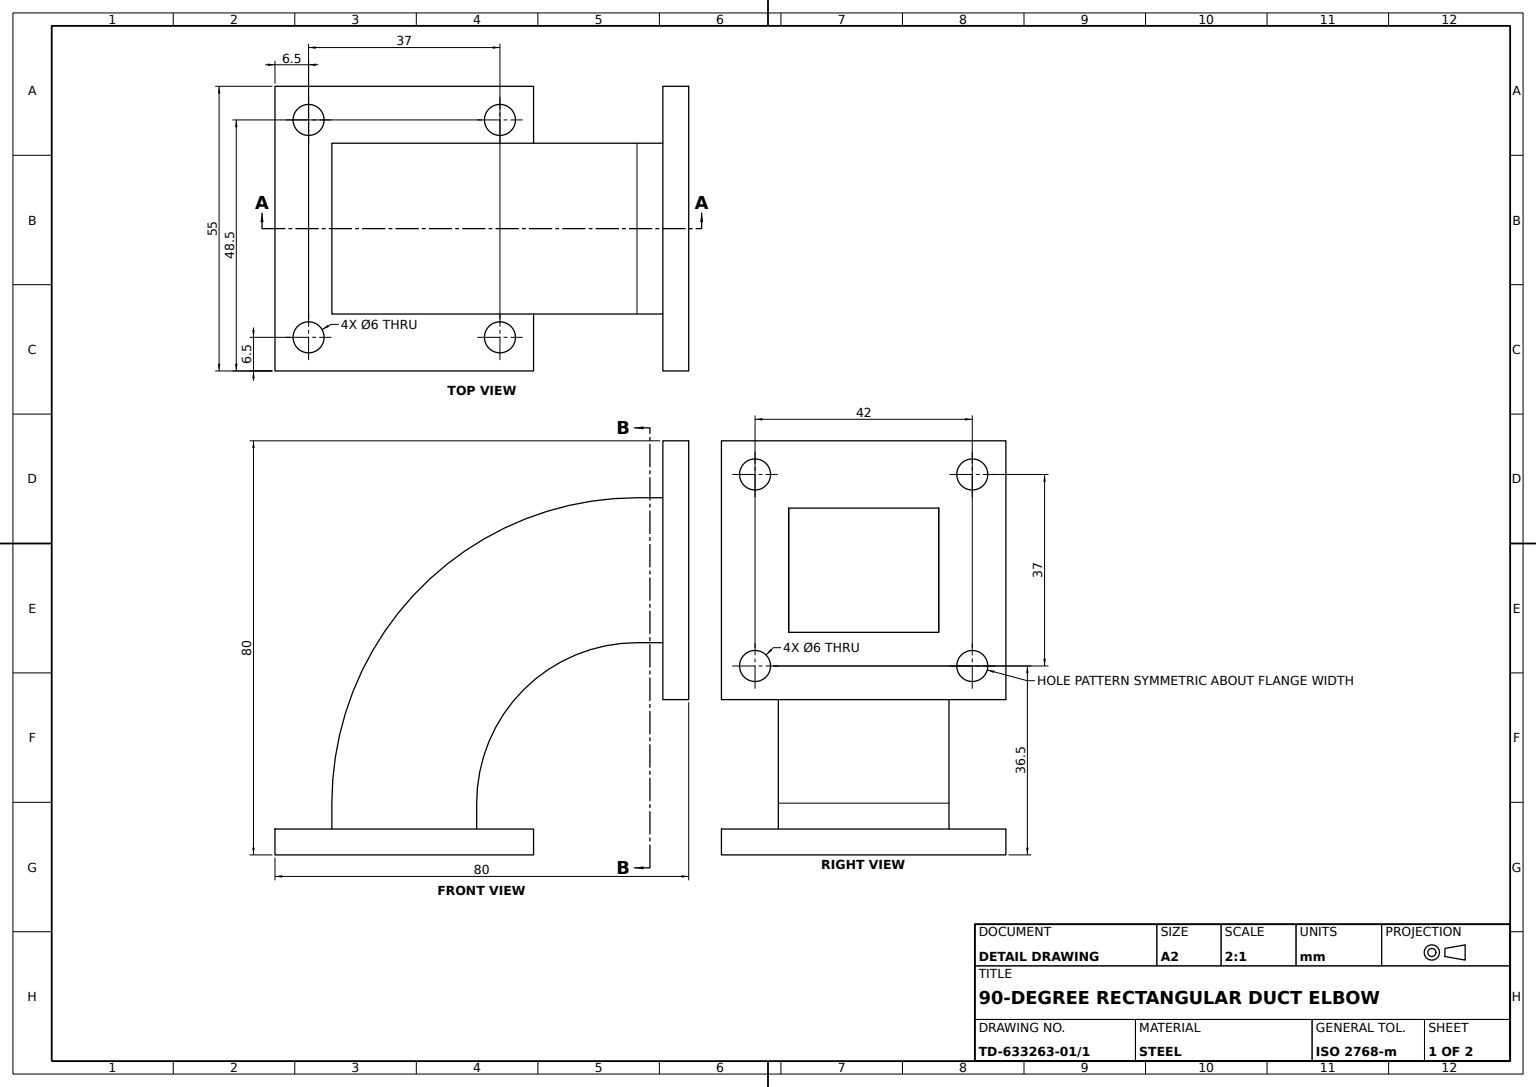
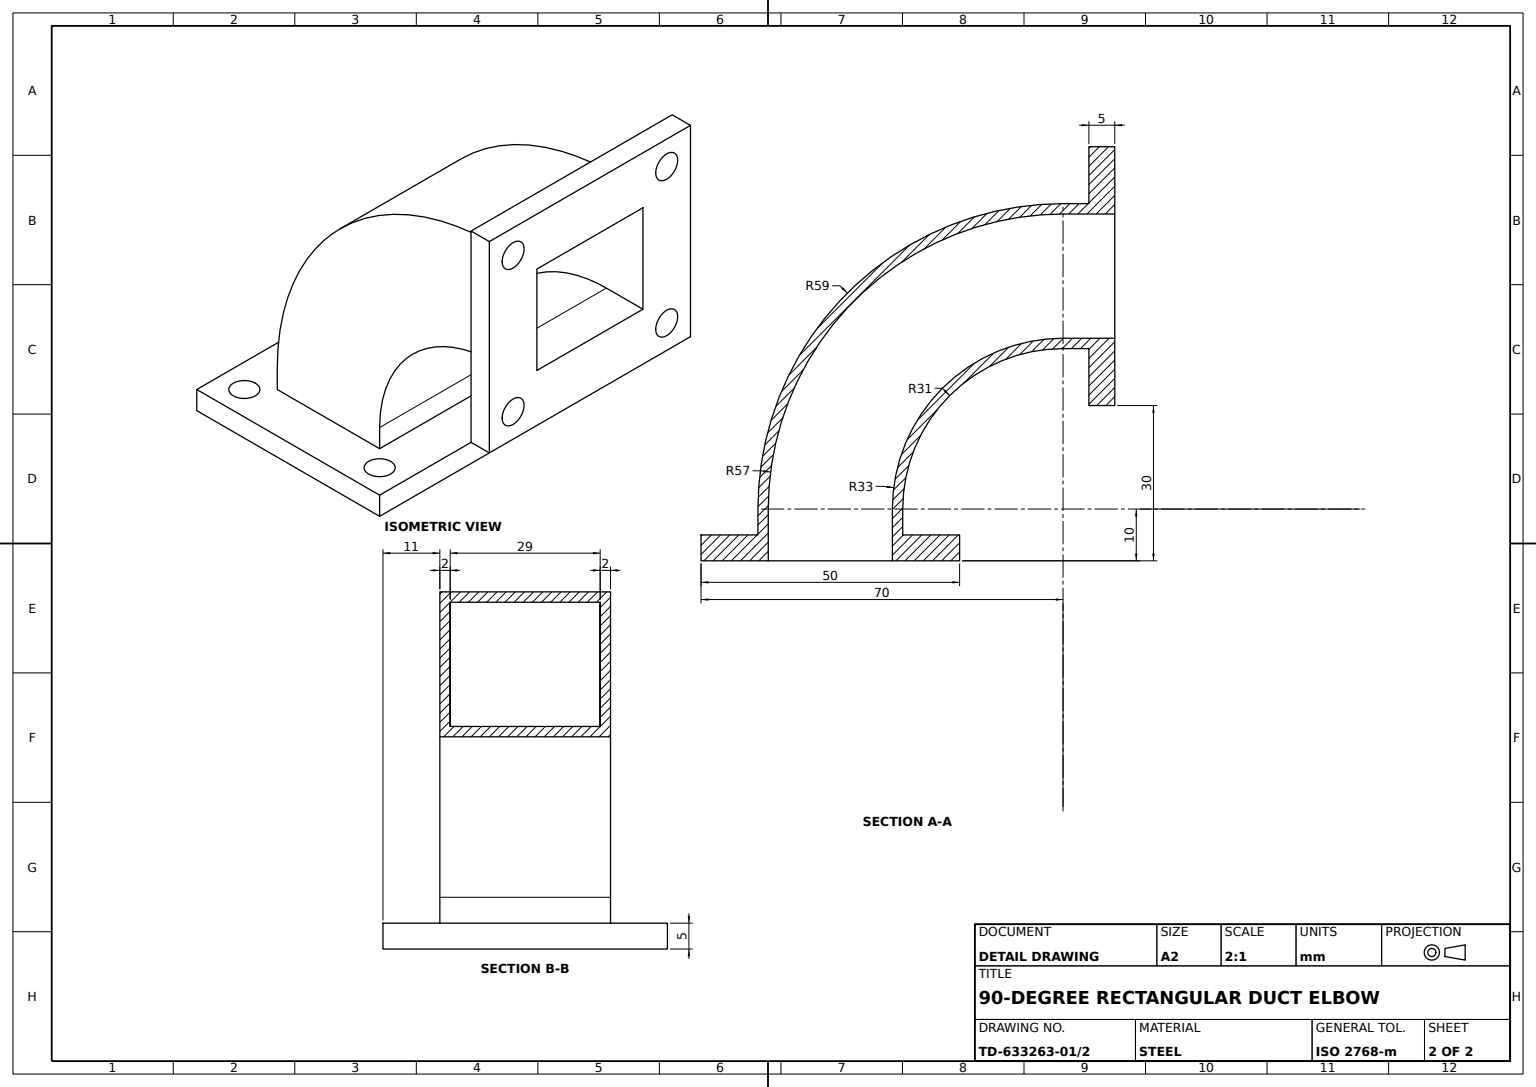
SolidWorks part; units mm, degrees
material "Plain Carbon Steel"
ref_plane "Front Plane" through (0, 0, 0) normal (0, 0, 1) x (1, 0, 0)
ref_plane "Top Plane" through (0, 0, 0) normal (0, 1, 0) x (1, 0, 0)
ref_plane "Right Plane" through (0, 0, 0) normal (1, 0, 0) x (0, 0, -1)
sketch "Inlet Flange Sketch" plane through (0, 0, 0) normal (1, 0, 0) x (0, 0, -1)
  line L1 (-14.5, 12) -> (14.5, 12)
  line L2 (-14.5, 12) -> (-14.5, -12)
  line L3 (-14.5, -12) -> (14.5, -12)
  line L4 (14.5, 12) -> (14.5, -12)
  line L5 (-14.5, 12) -> (14.5, -12) construction
  line L6 (-14.5, -12) -> (14.5, 12) construction
  line L7 (-27.5, 25) -> (27.5, 25)
  line L8 (-27.5, 25) -> (-27.5, -25)
  line L9 (-27.5, -25) -> (27.5, -25)
  line L10 (27.5, 25) -> (27.5, -25)
  line L11 (-27.5, 25) -> (27.5, -25) construction
  line L12 (-27.5, -25) -> (27.5, 25) construction
  circle A0 centre (-21, 18.5) radius 3
  circle A1 centre (21, 18.5) radius 3
  circle A2 centre (21, -18.5) radius 3
  circle A3 centre (-21, -18.5) radius 3
  point P0 (0, 0)
  point P5 (0, 0)
  dimension "D5" = 6
  dimension "D6" = 6
  dimension "D7" = 6
  dimension "D8" = 6
  dimension "D1" = 24
  dimension "D2" = 29
  dimension "D3" = 50
  dimension "D4" = 55
  dimension "D9" = 6.5
  dimension "D10" = 6.5
  dimension "D11" = 6.5
  dimension "D12" = 6.5
  dimension "D13" = 6.5
  dimension "D14" = 6.5
  dimension "D15" = 6.5
  dimension "D16" = 6.5
extrude "Inlet Flange 5mm" add sketch "Inlet Flange Sketch" along normal blind 5
ref_plane "Plane1" through (0, -50, 0) normal (0, 1, 0) x (1, 0, 0)
sketch "Outlet Flange Sketch" plane through (0, -50, 0) normal (0, 1, 0) x (1, 0, 0)
  line L0 (5, 27.5) -> (5, -27.5) construction
  line L1 (-75, 27.5) -> (-25, 27.5)
  line L2 (-75, 27.5) -> (-75, -27.5)
  line L3 (-75, -27.5) -> (-25, -27.5)
  line L4 (-25, 27.5) -> (-25, -27.5)
  line L5 (-75, 27.5) -> (-25, -27.5) construction
  line L6 (-75, -27.5) -> (-25, 27.5) construction
  line L8 (-62, 14.5) -> (-38, 14.5)
  line L9 (-62, 14.5) -> (-62, -14.5)
  line L10 (-62, -14.5) -> (-38, -14.5)
  line L11 (-38, 14.5) -> (-38, -14.5)
  line L12 (-62, 14.5) -> (-38, -14.5) construction
  line L13 (-62, -14.5) -> (-38, 14.5) construction
  circle A0 centre (-68.5, 21) radius 3
  circle A1 centre (-31.5, 21) radius 3
  circle A2 centre (-31.5, -21) radius 3
  circle A3 centre (-68.5, -21) radius 3
  point P0 (-50, 0)
  point P6 (-75, 0)
  point P9 (-50, 0)
  dimension "D6" = 6
  dimension "D7" = 6
  dimension "D8" = 6
  dimension "D9" = 6
  dimension "D1" = 55
  dimension "D2" = 50
  dimension "D3" = 80
  dimension "D4" = 29
  dimension "D5" = 24
  dimension "D10" = 6.5
  dimension "D11" = 6.5
  dimension "D12" = 6.5
  dimension "D13" = 6.5
  dimension "D14" = 6.5
  dimension "D15" = 6.5
  dimension "D16" = 6.5
  dimension "D17" = 6.5
extrude "Outlet Flange 5mm" add sketch "Outlet Flange Sketch" against normal blind 5 separate body
sketch "Bend Profile Sketch" plane through (0, -50, 0) normal (0, 1, 0) x (1, 0, 0)
  line L1 (-62, 14.5) -> (-38, 14.5)
  line L2 (-62, 14.5) -> (-62, -14.5)
  line L3 (-62, -14.5) -> (-38, -14.5)
  line L4 (-38, 14.5) -> (-38, -14.5)
ref_plane "Plane2" through (0, 0, 0) normal (0, 0, 1) x (1, 0, 0)
sketch "Bend Path R45 Sketch" plane through (0, 0, 0) normal (0, 0, 1) x (1, 0, 0)
  line L0 (-50, -50) -> (-50, -45)
  line L1 (-62, -50) -> (-38, -50) construction
  line L2 (-5, 0) -> (0, 0)
  arc A0 (-50, -45) -> (-5, 0) centre (-5, -45) cw
  dimension "D1" = 45
sweep "Elbow Bend Wall 2mm" add profiles "Bend Profile Sketch" path "Bend Path R45 Sketch" parameters "D1"=2
